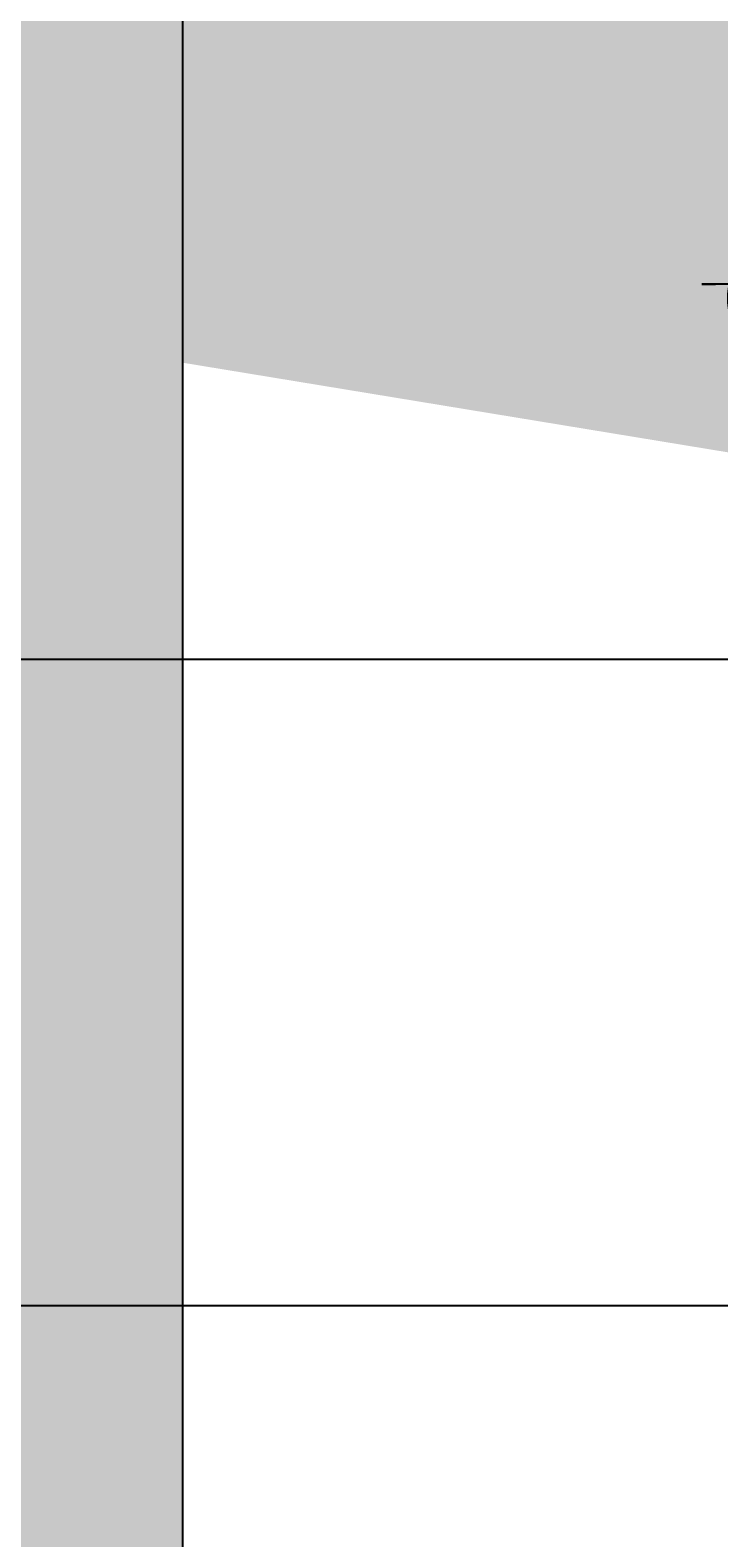
# Model space of a CAD drawing. Units: millimetres. Extents: x -22994 to 29398, y -19990 to 20176.
# Tile 52 of 135: x 198 to 216, y 25 to 65. Entities that reach past the tile are written whole.
import ezdxf
from ezdxf import colors
from ezdxf.entities.mleader import LeaderData, LeaderLine
from ezdxf.math import Vec2, Vec3

# ---------------------------------------------------------------- set-up
doc = ezdxf.new("R2010")
doc.units = ezdxf.units.MM
doc.header["$MEASUREMENT"] = 0
for name, color, linetype, lineweight in [('M-ANNO-TEXT', 7, 'Continuous', 25), ('M-DIMS', 2, 'Continuous', 18), ('M-EQPM', 7, 'Continuous', 25), ('M-EQPM-PATT', 7, 'Continuous', 18)]:
    doc.layers.add(name, color=color, linetype=linetype, lineweight=lineweight)
doc.styles.get("Standard").update_dxf_attribs({"font": 'arial.ttf'})
doc.dimstyles.get("Standard").update_dxf_attribs({"dimtxt": 0.18, "dimasz": 10000, "dimexe": 0.18, "dimexo": 0.0625, "dimgap": 0.09, "dimtad": 0, "dimtih": 1, "dimtoh": 1, "dimdec": 0, "dimzin": 0, "dimdsep": 46, "dimtxsty": 'Standard', "dimcen": 0.09, "dimadec": 0, "dimazin": 0, "dimtfac": 1, "dimtdec": 0, "dimtofl": 0, "dimtmove": 0, "dimatfit": 3, "dimfxl": 1, "dimtolj": 1, "dimtzin": 0, "dimlwd": 30, "dimarcsym": 0})

# ---------------------------------------------------------------- blocks, each defined once
blk = doc.blocks.new('*D2')
at = {"layer": 'Defpoints', "color": 0, "transparency": 16777216}
for p in [(6.677, 10.271), (290.852, 10.271), (290.852, -5.079)]:
    blk.add_point(p, dxfattribs=at)
at = {"layer": 'M-DIMS', "color": 0, "lineweight": -2, "transparency": 16777216}
for p, q in [((6.677, 10.209), (6.677, -5.259)), ((290.852, 10.209), (290.852, -5.259))]:
    blk.add_line(p, q, dxfattribs=at)
at = {"layer": 'M-DIMS', "color": 0, "lineweight": 30, "transparency": 16777216}
for p, q in [((-9993.323, -5.079), (-19993.323, -5.079)), ((10290.852, -5.079), (20290.852, -5.079))]:
    blk.add_line(p, q, dxfattribs=at)
at = {"layer": 'M-DIMS', "color": 0, "transparency": 16777216}
for points in [[(-9993.323, 1661.588), (-9993.323, -1671.745), (6.677, -5.079)], [(10290.852, 1661.588), (10290.852, -1671.745), (290.852, -5.079)]]:
    blk.add_solid(points, dxfattribs=at)
at = {"layer": 'M-DIMS', "color": 0, "transparency": 16777216, "insert": (148.765, -5.079), "char_height": 0.18, "attachment_point": 5}
blk.add_mtext('\\A1;284.2', dxfattribs=at)
blk = doc.blocks.new('*D3')
at = {"layer": 'Defpoints', "color": 0, "transparency": 16777216}
for p in [(110.265, 204.165), (110.265, 176.366), (95.833, 127.967)]:
    blk.add_point(p, dxfattribs=at)
at = {"layer": 'M-DIMS', "color": 0, "lineweight": -2, "transparency": 16777216}
for p, q in [((95.833, 128.03), (95.833, 204.345)), ((110.265, 176.429), (110.265, 204.345))]:
    blk.add_line(p, q, dxfattribs=at)
at = {"layer": 'M-DIMS', "color": 0, "lineweight": 30, "transparency": 16777216}
for p, q in [((-9904.167, 204.165), (-19904.167, 204.165)), ((10110.265, 204.165), (20110.265, 204.165))]:
    blk.add_line(p, q, dxfattribs=at)
at = {"layer": 'M-DIMS', "color": 0, "transparency": 16777216}
for points in [[(-9904.167, 1870.832), (-9904.167, -1462.501), (95.833, 204.165)], [(10110.265, 1870.832), (10110.265, -1462.501), (110.265, 204.165)]]:
    blk.add_solid(points, dxfattribs=at)
at = {"layer": 'M-DIMS', "color": 0, "transparency": 16777216, "insert": (103.049, 204.165), "char_height": 0.18, "attachment_point": 5}
blk.add_mtext('\\A1;14.432', dxfattribs=at)
blk = doc.blocks.new('*D4')
at = {"layer": 'Defpoints', "color": 0, "transparency": 16777216}
for p in [(116.265, 204.165), (110.265, 176.366), (116.265, 176.366)]:
    blk.add_point(p, dxfattribs=at)
at = {"layer": 'M-DIMS', "color": 0, "lineweight": -2, "transparency": 16777216}
for p, q in [((110.265, 176.429), (110.265, 204.345)), ((116.265, 176.429), (116.265, 204.345))]:
    blk.add_line(p, q, dxfattribs=at)
at = {"layer": 'M-DIMS', "color": 0, "lineweight": 30, "transparency": 16777216}
for p, q in [((-9889.735, 204.165), (-19889.735, 204.165)), ((10116.265, 204.165), (20116.265, 204.165))]:
    blk.add_line(p, q, dxfattribs=at)
at = {"layer": 'M-DIMS', "color": 0, "transparency": 16777216}
for points in [[(-9889.735, 1870.832), (-9889.735, -1462.501), (110.265, 204.165)], [(10116.265, 1870.832), (10116.265, -1462.501), (116.265, 204.165)]]:
    blk.add_solid(points, dxfattribs=at)
at = {"layer": 'M-DIMS', "color": 0, "transparency": 16777216, "insert": (113.265, 204.165), "char_height": 0.18, "attachment_point": 5}
blk.add_mtext('\\A1;6', dxfattribs=at)
blk = doc.blocks.new('*D5')
at = {"layer": 'Defpoints', "color": 0, "transparency": 16777216}
for p in [(181.265, 204.165), (116.265, 176.366), (181.265, 176.366)]:
    blk.add_point(p, dxfattribs=at)
at = {"layer": 'M-DIMS', "color": 0, "lineweight": -2, "transparency": 16777216}
for p, q in [((116.265, 176.429), (116.265, 204.345)), ((181.265, 176.429), (181.265, 204.345))]:
    blk.add_line(p, q, dxfattribs=at)
at = {"layer": 'M-DIMS', "color": 0, "lineweight": 30, "transparency": 16777216}
for p, q in [((-9883.735, 204.165), (-19883.735, 204.165)), ((10181.265, 204.165), (20181.265, 204.165))]:
    blk.add_line(p, q, dxfattribs=at)
at = {"layer": 'M-DIMS', "color": 0, "transparency": 16777216}
for points in [[(-9883.735, 1870.832), (-9883.735, -1462.501), (116.265, 204.165)], [(10181.265, 1870.832), (10181.265, -1462.501), (181.265, 204.165)]]:
    blk.add_solid(points, dxfattribs=at)
at = {"layer": 'M-DIMS', "color": 0, "transparency": 16777216, "insert": (148.765, 204.165), "char_height": 0.18, "attachment_point": 5}
blk.add_mtext('\\A1;65', dxfattribs=at)
blk = doc.blocks.new('*D6')
at = {"layer": 'Defpoints', "color": 0, "transparency": 16777216}
for p in [(187.265, 204.165), (181.265, 176.366), (187.265, 176.366)]:
    blk.add_point(p, dxfattribs=at)
at = {"layer": 'M-DIMS', "color": 0, "lineweight": -2, "transparency": 16777216}
for p, q in [((181.265, 176.429), (181.265, 204.345)), ((187.265, 176.429), (187.265, 204.345))]:
    blk.add_line(p, q, dxfattribs=at)
at = {"layer": 'M-DIMS', "color": 0, "lineweight": 30, "transparency": 16777216}
for p, q in [((-9818.735, 204.165), (-19818.735, 204.165)), ((10187.265, 204.165), (20187.265, 204.165))]:
    blk.add_line(p, q, dxfattribs=at)
at = {"layer": 'M-DIMS', "color": 0, "transparency": 16777216}
for points in [[(-9818.735, 1870.832), (-9818.735, -1462.501), (181.265, 204.165)], [(10187.265, 1870.832), (10187.265, -1462.501), (187.265, 204.165)]]:
    blk.add_solid(points, dxfattribs=at)
at = {"layer": 'M-DIMS', "color": 0, "transparency": 16777216, "insert": (184.265, 204.165), "char_height": 0.18, "attachment_point": 5}
blk.add_mtext('\\A1;6', dxfattribs=at)
blk = doc.blocks.new('*D7')
at = {"layer": 'Defpoints', "color": 0, "transparency": 16777216}
for p in [(201.697, 204.165), (187.265, 176.366), (201.697, 127.967)]:
    blk.add_point(p, dxfattribs=at)
at = {"layer": 'M-DIMS', "color": 0, "lineweight": -2, "transparency": 16777216}
for p, q in [((187.265, 176.429), (187.265, 204.345)), ((201.697, 128.03), (201.697, 204.345))]:
    blk.add_line(p, q, dxfattribs=at)
at = {"layer": 'M-DIMS', "color": 0, "lineweight": 30, "transparency": 16777216}
for p, q in [((-9812.735, 204.165), (-19812.735, 204.165)), ((10201.697, 204.165), (20201.697, 204.165))]:
    blk.add_line(p, q, dxfattribs=at)
at = {"layer": 'M-DIMS', "color": 0, "transparency": 16777216}
for points in [[(-9812.735, 1870.832), (-9812.735, -1462.501), (187.265, 204.165)], [(10201.697, 1870.832), (10201.697, -1462.501), (201.697, 204.165)]]:
    blk.add_solid(points, dxfattribs=at)
at = {"layer": 'M-DIMS', "color": 0, "transparency": 16777216, "insert": (194.481, 204.165), "char_height": 0.18, "attachment_point": 5}
blk.add_mtext('\\A1;14.432', dxfattribs=at)
blk = doc.blocks.new('*D8')
at = {"layer": 'Defpoints', "color": 0, "transparency": 16777216}
for p in [(227.648, 204.165), (227.648, 146.73), (201.697, 127.967)]:
    blk.add_point(p, dxfattribs=at)
at = {"layer": 'M-DIMS', "color": 0, "lineweight": -2, "transparency": 16777216}
for p, q in [((201.697, 128.03), (201.697, 204.345)), ((227.648, 146.792), (227.648, 204.345))]:
    blk.add_line(p, q, dxfattribs=at)
at = {"layer": 'M-DIMS', "color": 0, "lineweight": 30, "transparency": 16777216}
for p, q in [((-9798.303, 204.165), (-19798.303, 204.165)), ((10227.648, 204.165), (20227.648, 204.165))]:
    blk.add_line(p, q, dxfattribs=at)
at = {"layer": 'M-DIMS', "color": 0, "transparency": 16777216}
for points in [[(-9798.303, 1870.832), (-9798.303, -1462.501), (201.697, 204.165)], [(10227.648, 1870.832), (10227.648, -1462.501), (227.648, 204.165)]]:
    blk.add_solid(points, dxfattribs=at)
at = {"layer": 'M-DIMS', "color": 0, "transparency": 16777216, "insert": (214.673, 204.165), "char_height": 0.18, "attachment_point": 5}
blk.add_mtext('\\A1;25.95', dxfattribs=at)
blk = doc.blocks.new('*D9')
at = {"layer": 'Defpoints', "color": 0, "transparency": 16777216}
for p in [(187.265, 176.366), (306.202, 176.366), (290.852, 10.271)]:
    blk.add_point(p, dxfattribs=at)
at = {"layer": 'M-DIMS', "color": 0, "lineweight": 30, "transparency": 16777216}
for p, q in [((306.202, 10176.366), (306.202, 20176.366)), ((306.202, -9989.729), (306.202, -19989.729))]:
    blk.add_line(p, q, dxfattribs=at)
at = {"layer": 'M-DIMS', "color": 0, "lineweight": -2, "transparency": 16777216}
for p, q in [((187.327, 176.366), (306.382, 176.366)), ((290.915, 10.271), (306.382, 10.271))]:
    blk.add_line(p, q, dxfattribs=at)
at = {"layer": 'M-DIMS', "color": 0, "transparency": 16777216}
for points in [[(-1360.465, 10176.366), (1972.869, 10176.366), (306.202, 176.366)], [(-1360.465, -9989.729), (1972.869, -9989.729), (306.202, 10.271)]]:
    blk.add_solid(points, dxfattribs=at)
at = {"layer": 'M-DIMS', "color": 0, "transparency": 16777216, "insert": (306.202, 93.319), "char_height": 0.18, "attachment_point": 5}
blk.add_mtext('\\A1;166.1', dxfattribs=at)
blk = doc.blocks.new('*D10')
at = {"layer": 'Defpoints', "color": 0, "transparency": 16777216}
for p in [(125.65, 136.071), (133.346, 136.071), (133.346, -5.079)]:
    blk.add_point(p, dxfattribs=at)
at = {"layer": 'M-DIMS', "color": 0, "lineweight": -2, "transparency": 16777216}
for p, q in [((125.65, 136.009), (125.65, -5.259)), ((133.346, 136.009), (133.346, -5.259))]:
    blk.add_line(p, q, dxfattribs=at)
at = {"layer": 'M-DIMS', "color": 0, "lineweight": 30, "transparency": 16777216}
for p, q in [((-9874.35, -5.079), (-19874.35, -5.079)), ((10133.346, -5.079), (20133.346, -5.079))]:
    blk.add_line(p, q, dxfattribs=at)
at = {"layer": 'M-DIMS', "color": 0, "transparency": 16777216}
for points in [[(-9874.35, 1661.588), (-9874.35, -1671.745), (125.65, -5.079)], [(10133.346, 1661.588), (10133.346, -1671.745), (133.346, -5.079)]]:
    blk.add_solid(points, dxfattribs=at)
at = {"layer": 'M-DIMS', "color": 0, "transparency": 16777216, "insert": (129.498, -5.079), "char_height": 0.18, "attachment_point": 5}
blk.add_mtext('\\A1;7.696', dxfattribs=at)
blk = doc.blocks.new('*D11')
at = {"layer": 'Defpoints', "color": 0, "transparency": 16777216}
for p in [(133.346, 136.071), (135.65, 136.071), (135.65, -5.079)]:
    blk.add_point(p, dxfattribs=at)
at = {"layer": 'M-DIMS', "color": 0, "lineweight": -2, "transparency": 16777216}
for p, q in [((133.346, 136.009), (133.346, -5.259)), ((135.65, 136.009), (135.65, -5.259))]:
    blk.add_line(p, q, dxfattribs=at)
at = {"layer": 'M-DIMS', "color": 0, "lineweight": 30, "transparency": 16777216}
for p, q in [((-9866.654, -5.079), (-19866.654, -5.079)), ((10135.65, -5.079), (20135.65, -5.079))]:
    blk.add_line(p, q, dxfattribs=at)
at = {"layer": 'M-DIMS', "color": 0, "transparency": 16777216}
for points in [[(-9866.654, 1661.588), (-9866.654, -1671.745), (133.346, -5.079)], [(10135.65, 1661.588), (10135.65, -1671.745), (135.65, -5.079)]]:
    blk.add_solid(points, dxfattribs=at)
at = {"layer": 'M-DIMS', "color": 0, "transparency": 16777216, "insert": (134.498, -5.079), "char_height": 0.18, "attachment_point": 5}
blk.add_mtext('\\A1;2.304', dxfattribs=at)
blk = doc.blocks.new('*D12')
at = {"layer": 'Defpoints', "color": 0, "transparency": 16777216}
for p in [(135.65, 136.071), (145.65, 136.071), (145.65, -5.079)]:
    blk.add_point(p, dxfattribs=at)
at = {"layer": 'M-DIMS', "color": 0, "lineweight": -2, "transparency": 16777216}
for p, q in [((135.65, 136.009), (135.65, -5.259)), ((145.65, 136.009), (145.65, -5.259))]:
    blk.add_line(p, q, dxfattribs=at)
at = {"layer": 'M-DIMS', "color": 0, "lineweight": 30, "transparency": 16777216}
for p, q in [((-9864.35, -5.079), (-19864.35, -5.079)), ((10145.65, -5.079), (20145.65, -5.079))]:
    blk.add_line(p, q, dxfattribs=at)
at = {"layer": 'M-DIMS', "color": 0, "transparency": 16777216}
for points in [[(-9864.35, 1661.588), (-9864.35, -1671.745), (135.65, -5.079)], [(10145.65, 1661.588), (10145.65, -1671.745), (145.65, -5.079)]]:
    blk.add_solid(points, dxfattribs=at)
at = {"layer": 'M-DIMS', "color": 0, "transparency": 16777216, "insert": (140.65, -5.079), "char_height": 0.18, "attachment_point": 5}
blk.add_mtext('\\A1;10', dxfattribs=at)
blk = doc.blocks.new('*D13')
at = {"layer": 'Defpoints', "color": 0, "transparency": 16777216}
for p in [(145.65, 136.071), (155.65, 136.071), (155.65, -5.079)]:
    blk.add_point(p, dxfattribs=at)
at = {"layer": 'M-DIMS', "color": 0, "lineweight": -2, "transparency": 16777216}
for p, q in [((145.65, 136.009), (145.65, -5.259)), ((155.65, 136.009), (155.65, -5.259))]:
    blk.add_line(p, q, dxfattribs=at)
at = {"layer": 'M-DIMS', "color": 0, "lineweight": 30, "transparency": 16777216}
for p, q in [((-9854.35, -5.079), (-19854.35, -5.079)), ((10155.65, -5.079), (20155.65, -5.079))]:
    blk.add_line(p, q, dxfattribs=at)
at = {"layer": 'M-DIMS', "color": 0, "transparency": 16777216}
for points in [[(-9854.35, 1661.588), (-9854.35, -1671.745), (145.65, -5.079)], [(10155.65, 1661.588), (10155.65, -1671.745), (155.65, -5.079)]]:
    blk.add_solid(points, dxfattribs=at)
at = {"layer": 'M-DIMS', "color": 0, "transparency": 16777216, "insert": (150.65, -5.079), "char_height": 0.18, "attachment_point": 5}
blk.add_mtext('\\A1;10', dxfattribs=at)
blk = doc.blocks.new('*D14')
at = {"layer": 'Defpoints', "color": 0, "transparency": 16777216}
for p in [(155.65, 136.071), (165.65, 136.071), (165.65, -5.079)]:
    blk.add_point(p, dxfattribs=at)
at = {"layer": 'M-DIMS', "color": 0, "lineweight": -2, "transparency": 16777216}
for p, q in [((155.65, 136.009), (155.65, -5.259)), ((165.65, 136.009), (165.65, -5.259))]:
    blk.add_line(p, q, dxfattribs=at)
at = {"layer": 'M-DIMS', "color": 0, "lineweight": 30, "transparency": 16777216}
for p, q in [((-9844.35, -5.079), (-19844.35, -5.079)), ((10165.65, -5.079), (20165.65, -5.079))]:
    blk.add_line(p, q, dxfattribs=at)
at = {"layer": 'M-DIMS', "color": 0, "transparency": 16777216}
for points in [[(-9844.35, 1661.588), (-9844.35, -1671.745), (155.65, -5.079)], [(10165.65, 1661.588), (10165.65, -1671.745), (165.65, -5.079)]]:
    blk.add_solid(points, dxfattribs=at)
at = {"layer": 'M-DIMS', "color": 0, "transparency": 16777216, "insert": (160.65, -5.079), "char_height": 0.18, "attachment_point": 5}
blk.add_mtext('\\A1;10', dxfattribs=at)
blk = doc.blocks.new('*D15')
at = {"layer": 'Defpoints', "color": 0, "transparency": 16777216}
for p in [(173.346, 154.788), (173.346, 136.071), (306.202, 136.071)]:
    blk.add_point(p, dxfattribs=at)
at = {"layer": 'M-DIMS', "color": 0, "lineweight": 30, "transparency": 16777216}
for p, q in [((306.202, 10154.788), (306.202, 20154.788)), ((306.202, -9863.929), (306.202, -19863.929))]:
    blk.add_line(p, q, dxfattribs=at)
at = {"layer": 'M-DIMS', "color": 0, "lineweight": -2, "transparency": 16777216}
for p, q in [((173.408, 154.788), (306.382, 154.788)), ((173.408, 136.071), (306.382, 136.071))]:
    blk.add_line(p, q, dxfattribs=at)
at = {"layer": 'M-DIMS', "color": 0, "transparency": 16777216}
for points in [[(-1360.465, 10154.788), (1972.869, 10154.788), (306.202, 154.788)], [(-1360.465, -9863.929), (1972.869, -9863.929), (306.202, 136.071)]]:
    blk.add_solid(points, dxfattribs=at)
at = {"layer": 'M-DIMS', "color": 0, "transparency": 16777216, "insert": (306.202, 145.43), "char_height": 0.18, "attachment_point": 5}
blk.add_mtext('\\A1;18.717', dxfattribs=at)
blk = doc.blocks.new('*D16')
at = {"layer": 'Defpoints', "color": 0, "transparency": 16777216}
for p in [(120.17, 204.165), (110.466, 48.035), (120.17, 48.035)]:
    blk.add_point(p, dxfattribs=at)
at = {"layer": 'M-DIMS', "color": 0, "lineweight": -2, "transparency": 16777216}
for p, q in [((110.466, 48.097), (110.466, 204.345)), ((120.17, 48.097), (120.17, 204.345))]:
    blk.add_line(p, q, dxfattribs=at)
at = {"layer": 'M-DIMS', "color": 0, "lineweight": 30, "transparency": 16777216}
for p, q in [((-9889.534, 204.165), (-19889.534, 204.165)), ((10120.17, 204.165), (20120.17, 204.165))]:
    blk.add_line(p, q, dxfattribs=at)
at = {"layer": 'M-DIMS', "color": 0, "transparency": 16777216}
for points in [[(-9889.534, 1870.832), (-9889.534, -1462.501), (110.466, 204.165)], [(10120.17, 1870.832), (10120.17, -1462.501), (120.17, 204.165)]]:
    blk.add_solid(points, dxfattribs=at)
at = {"layer": 'M-DIMS', "color": 0, "transparency": 16777216, "insert": (115.318, 204.165), "char_height": 0.18, "attachment_point": 5}
blk.add_mtext('\\A1;9.704', dxfattribs=at)
blk = doc.blocks.new('*D17')
at = {"layer": 'Defpoints', "color": 0, "transparency": 16777216}
for p in [(126.17, 204.165), (120.17, 48.035), (126.17, 48.035)]:
    blk.add_point(p, dxfattribs=at)
at = {"layer": 'M-DIMS', "color": 0, "lineweight": -2, "transparency": 16777216}
for p, q in [((120.17, 48.097), (120.17, 204.345)), ((126.17, 48.097), (126.17, 204.345))]:
    blk.add_line(p, q, dxfattribs=at)
at = {"layer": 'M-DIMS', "color": 0, "lineweight": 30, "transparency": 16777216}
for p, q in [((-9879.83, 204.165), (-19879.83, 204.165)), ((10126.17, 204.165), (20126.17, 204.165))]:
    blk.add_line(p, q, dxfattribs=at)
at = {"layer": 'M-DIMS', "color": 0, "transparency": 16777216}
for points in [[(-9879.83, 1870.832), (-9879.83, -1462.501), (120.17, 204.165)], [(10126.17, 1870.832), (10126.17, -1462.501), (126.17, 204.165)]]:
    blk.add_solid(points, dxfattribs=at)
at = {"layer": 'M-DIMS', "color": 0, "transparency": 16777216, "insert": (123.17, 204.165), "char_height": 0.18, "attachment_point": 5}
blk.add_mtext('\\A1;6', dxfattribs=at)
blk = doc.blocks.new('*D18')
at = {"layer": 'Defpoints', "color": 0, "transparency": 16777216}
for p in [(132.17, 204.165), (126.17, 48.035), (132.17, 48.035)]:
    blk.add_point(p, dxfattribs=at)
at = {"layer": 'M-DIMS', "color": 0, "lineweight": -2, "transparency": 16777216}
for p, q in [((126.17, 48.097), (126.17, 204.345)), ((132.17, 48.097), (132.17, 204.345))]:
    blk.add_line(p, q, dxfattribs=at)
at = {"layer": 'M-DIMS', "color": 0, "lineweight": 30, "transparency": 16777216}
for p, q in [((-9873.83, 204.165), (-19873.83, 204.165)), ((10132.17, 204.165), (20132.17, 204.165))]:
    blk.add_line(p, q, dxfattribs=at)
at = {"layer": 'M-DIMS', "color": 0, "transparency": 16777216}
for points in [[(-9873.83, 1870.832), (-9873.83, -1462.501), (126.17, 204.165)], [(10132.17, 1870.832), (10132.17, -1462.501), (132.17, 204.165)]]:
    blk.add_solid(points, dxfattribs=at)
at = {"layer": 'M-DIMS', "color": 0, "transparency": 16777216, "insert": (129.17, 204.165), "char_height": 0.18, "attachment_point": 5}
blk.add_mtext('\\A1;6', dxfattribs=at)
blk = doc.blocks.new('*D19')
at = {"layer": 'Defpoints', "color": 0, "transparency": 16777216}
for p in [(138.17, 204.165), (132.17, 48.035), (138.17, 48.035)]:
    blk.add_point(p, dxfattribs=at)
at = {"layer": 'M-DIMS', "color": 0, "lineweight": -2, "transparency": 16777216}
for p, q in [((132.17, 48.097), (132.17, 204.345)), ((138.17, 48.097), (138.17, 204.345))]:
    blk.add_line(p, q, dxfattribs=at)
at = {"layer": 'M-DIMS', "color": 0, "lineweight": 30, "transparency": 16777216}
for p, q in [((-9867.83, 204.165), (-19867.83, 204.165)), ((10138.17, 204.165), (20138.17, 204.165))]:
    blk.add_line(p, q, dxfattribs=at)
at = {"layer": 'M-DIMS', "color": 0, "transparency": 16777216}
for points in [[(-9867.83, 1870.832), (-9867.83, -1462.501), (132.17, 204.165)], [(10138.17, 1870.832), (10138.17, -1462.501), (138.17, 204.165)]]:
    blk.add_solid(points, dxfattribs=at)
at = {"layer": 'M-DIMS', "color": 0, "transparency": 16777216, "insert": (135.17, 204.165), "char_height": 0.18, "attachment_point": 5}
blk.add_mtext('\\A1;6', dxfattribs=at)
blk = doc.blocks.new('*D20')
at = {"layer": 'Defpoints', "color": 0, "transparency": 16777216}
for p in [(144.17, 204.165), (138.17, 48.035), (144.17, 48.035)]:
    blk.add_point(p, dxfattribs=at)
at = {"layer": 'M-DIMS', "color": 0, "lineweight": -2, "transparency": 16777216}
for p, q in [((138.17, 48.097), (138.17, 204.345)), ((144.17, 48.097), (144.17, 204.345))]:
    blk.add_line(p, q, dxfattribs=at)
at = {"layer": 'M-DIMS', "color": 0, "lineweight": 30, "transparency": 16777216}
for p, q in [((-9861.83, 204.165), (-19861.83, 204.165)), ((10144.17, 204.165), (20144.17, 204.165))]:
    blk.add_line(p, q, dxfattribs=at)
at = {"layer": 'M-DIMS', "color": 0, "transparency": 16777216}
for points in [[(-9861.83, 1870.832), (-9861.83, -1462.501), (138.17, 204.165)], [(10144.17, 1870.832), (10144.17, -1462.501), (144.17, 204.165)]]:
    blk.add_solid(points, dxfattribs=at)
at = {"layer": 'M-DIMS', "color": 0, "transparency": 16777216, "insert": (141.17, 204.165), "char_height": 0.18, "attachment_point": 5}
blk.add_mtext('\\A1;6', dxfattribs=at)
blk = doc.blocks.new('*D21')
at = {"layer": 'Defpoints', "color": 0, "transparency": 16777216}
for p in [(149.116, 204.165), (144.17, 48.035), (149.116, 48.035)]:
    blk.add_point(p, dxfattribs=at)
at = {"layer": 'M-DIMS', "color": 0, "lineweight": -2, "transparency": 16777216}
for p, q in [((144.17, 48.097), (144.17, 204.345)), ((149.116, 48.097), (149.116, 204.345))]:
    blk.add_line(p, q, dxfattribs=at)
at = {"layer": 'M-DIMS', "color": 0, "lineweight": 30, "transparency": 16777216}
for p, q in [((-9855.83, 204.165), (-19855.83, 204.165)), ((10149.116, 204.165), (20149.116, 204.165))]:
    blk.add_line(p, q, dxfattribs=at)
at = {"layer": 'M-DIMS', "color": 0, "transparency": 16777216}
for points in [[(-9855.83, 1870.832), (-9855.83, -1462.501), (144.17, 204.165)], [(10149.116, 1870.832), (10149.116, -1462.501), (149.116, 204.165)]]:
    blk.add_solid(points, dxfattribs=at)
at = {"layer": 'M-DIMS', "color": 0, "transparency": 16777216, "insert": (146.643, 204.165), "char_height": 0.18, "attachment_point": 5}
blk.add_mtext('\\A1;4.945', dxfattribs=at)
blk = doc.blocks.new('*D22')
at = {"layer": 'Defpoints', "color": 0, "transparency": 16777216}
for p in [(149.116, 30.99), (155.116, 30.99), (155.116, -5.079)]:
    blk.add_point(p, dxfattribs=at)
at = {"layer": 'M-DIMS', "color": 0, "lineweight": -2, "transparency": 16777216}
for p, q in [((149.116, 30.927), (149.116, -5.259)), ((155.116, 30.927), (155.116, -5.259))]:
    blk.add_line(p, q, dxfattribs=at)
at = {"layer": 'M-DIMS', "color": 0, "lineweight": 30, "transparency": 16777216}
for p, q in [((-9850.884, -5.079), (-19850.884, -5.079)), ((10155.116, -5.079), (20155.116, -5.079))]:
    blk.add_line(p, q, dxfattribs=at)
at = {"layer": 'M-DIMS', "color": 0, "transparency": 16777216}
for points in [[(-9850.884, 1661.588), (-9850.884, -1671.745), (149.116, -5.079)], [(10155.116, 1661.588), (10155.116, -1671.745), (155.116, -5.079)]]:
    blk.add_solid(points, dxfattribs=at)
at = {"layer": 'M-DIMS', "color": 0, "transparency": 16777216, "insert": (152.116, -5.079), "char_height": 0.18, "attachment_point": 5}
blk.add_mtext('\\A1;6', dxfattribs=at)
blk = doc.blocks.new('*D23')
at = {"layer": 'Defpoints', "color": 0, "transparency": 16777216}
for p in [(155.116, 30.99), (161.116, 30.99), (161.116, -5.079)]:
    blk.add_point(p, dxfattribs=at)
at = {"layer": 'M-DIMS', "color": 0, "lineweight": -2, "transparency": 16777216}
for p, q in [((155.116, 30.927), (155.116, -5.259)), ((161.116, 30.927), (161.116, -5.259))]:
    blk.add_line(p, q, dxfattribs=at)
at = {"layer": 'M-DIMS', "color": 0, "lineweight": 30, "transparency": 16777216}
for p, q in [((-9844.884, -5.079), (-19844.884, -5.079)), ((10161.116, -5.079), (20161.116, -5.079))]:
    blk.add_line(p, q, dxfattribs=at)
at = {"layer": 'M-DIMS', "color": 0, "transparency": 16777216}
for points in [[(-9844.884, 1661.588), (-9844.884, -1671.745), (155.116, -5.079)], [(10161.116, 1661.588), (10161.116, -1671.745), (161.116, -5.079)]]:
    blk.add_solid(points, dxfattribs=at)
at = {"layer": 'M-DIMS', "color": 0, "transparency": 16777216, "insert": (158.116, -5.079), "char_height": 0.18, "attachment_point": 5}
blk.add_mtext('\\A1;6', dxfattribs=at)
blk = doc.blocks.new('*D24')
at = {"layer": 'Defpoints', "color": 0, "transparency": 16777216}
for p in [(161.116, 30.99), (166.439, 30.99), (166.439, -5.079)]:
    blk.add_point(p, dxfattribs=at)
at = {"layer": 'M-DIMS', "color": 0, "lineweight": -2, "transparency": 16777216}
for p, q in [((161.116, 30.927), (161.116, -5.259)), ((166.439, 30.927), (166.439, -5.259))]:
    blk.add_line(p, q, dxfattribs=at)
at = {"layer": 'M-DIMS', "color": 0, "lineweight": 30, "transparency": 16777216}
for p, q in [((-9838.884, -5.079), (-19838.884, -5.079)), ((10166.439, -5.079), (20166.439, -5.079))]:
    blk.add_line(p, q, dxfattribs=at)
at = {"layer": 'M-DIMS', "color": 0, "transparency": 16777216}
for points in [[(-9838.884, 1661.588), (-9838.884, -1671.745), (161.116, -5.079)], [(10166.439, 1661.588), (10166.439, -1671.745), (166.439, -5.079)]]:
    blk.add_solid(points, dxfattribs=at)
at = {"layer": 'M-DIMS', "color": 0, "transparency": 16777216, "insert": (163.777, -5.079), "char_height": 0.18, "attachment_point": 5}
blk.add_mtext('\\A1;5.323', dxfattribs=at)
blk = doc.blocks.new('*D25')
at = {"layer": 'Defpoints', "color": 0, "transparency": 16777216}
for p in [(166.439, 30.99), (172.439, 30.99), (172.439, -5.079)]:
    blk.add_point(p, dxfattribs=at)
at = {"layer": 'M-DIMS', "color": 0, "lineweight": -2, "transparency": 16777216}
for p, q in [((166.439, 30.927), (166.439, -5.259)), ((172.439, 30.927), (172.439, -5.259))]:
    blk.add_line(p, q, dxfattribs=at)
at = {"layer": 'M-DIMS', "color": 0, "lineweight": 30, "transparency": 16777216}
for p, q in [((-9833.561, -5.079), (-19833.561, -5.079)), ((10172.439, -5.079), (20172.439, -5.079))]:
    blk.add_line(p, q, dxfattribs=at)
at = {"layer": 'M-DIMS', "color": 0, "transparency": 16777216}
for points in [[(-9833.561, 1661.588), (-9833.561, -1671.745), (166.439, -5.079)], [(10172.439, 1661.588), (10172.439, -1671.745), (172.439, -5.079)]]:
    blk.add_solid(points, dxfattribs=at)
at = {"layer": 'M-DIMS', "color": 0, "transparency": 16777216, "insert": (169.439, -5.079), "char_height": 0.18, "attachment_point": 5}
blk.add_mtext('\\A1;6', dxfattribs=at)
blk = doc.blocks.new('*D26')
at = {"layer": 'Defpoints', "color": 0, "transparency": 16777216}
for p in [(172.439, 30.99), (178.439, 30.99), (178.439, -5.079)]:
    blk.add_point(p, dxfattribs=at)
at = {"layer": 'M-DIMS', "color": 0, "lineweight": -2, "transparency": 16777216}
for p, q in [((172.439, 30.927), (172.439, -5.259)), ((178.439, 30.927), (178.439, -5.259))]:
    blk.add_line(p, q, dxfattribs=at)
at = {"layer": 'M-DIMS', "color": 0, "lineweight": 30, "transparency": 16777216}
for p, q in [((-9827.561, -5.079), (-19827.561, -5.079)), ((10178.439, -5.079), (20178.439, -5.079))]:
    blk.add_line(p, q, dxfattribs=at)
at = {"layer": 'M-DIMS', "color": 0, "transparency": 16777216}
for points in [[(-9827.561, 1661.588), (-9827.561, -1671.745), (172.439, -5.079)], [(10178.439, 1661.588), (10178.439, -1671.745), (178.439, -5.079)]]:
    blk.add_solid(points, dxfattribs=at)
at = {"layer": 'M-DIMS', "color": 0, "transparency": 16777216, "insert": (175.439, -5.079), "char_height": 0.18, "attachment_point": 5}
blk.add_mtext('\\A1;6', dxfattribs=at)
blk = doc.blocks.new('*D27')
at = {"layer": 'Defpoints', "color": 0, "transparency": 16777216}
for p in [(178.439, 30.99), (188.117, 30.99), (188.117, -5.079)]:
    blk.add_point(p, dxfattribs=at)
at = {"layer": 'M-DIMS', "color": 0, "lineweight": -2, "transparency": 16777216}
for p, q in [((178.439, 30.927), (178.439, -5.259)), ((188.117, 30.927), (188.117, -5.259))]:
    blk.add_line(p, q, dxfattribs=at)
at = {"layer": 'M-DIMS', "color": 0, "lineweight": 30, "transparency": 16777216}
for p, q in [((-9821.561, -5.079), (-19821.561, -5.079)), ((10188.117, -5.079), (20188.117, -5.079))]:
    blk.add_line(p, q, dxfattribs=at)
at = {"layer": 'M-DIMS', "color": 0, "transparency": 16777216}
for points in [[(-9821.561, 1661.588), (-9821.561, -1671.745), (178.439, -5.079)], [(10188.117, 1661.588), (10188.117, -1671.745), (188.117, -5.079)]]:
    blk.add_solid(points, dxfattribs=at)
at = {"layer": 'M-DIMS', "color": 0, "transparency": 16777216, "insert": (183.278, -5.079), "char_height": 0.18, "attachment_point": 5}
blk.add_mtext('\\A1;9.679', dxfattribs=at)
blk = doc.blocks.new('*D28')
at = {"layer": 'Defpoints', "color": 0, "transparency": 16777216}
for p in [(188.117, 48.035), (306.202, 48.035), (188.117, 30.99)]:
    blk.add_point(p, dxfattribs=at)
at = {"layer": 'M-DIMS', "color": 0, "lineweight": 30, "transparency": 16777216}
for p, q in [((306.202, 10048.035), (306.202, 20048.035)), ((306.202, -9969.01), (306.202, -19969.01))]:
    blk.add_line(p, q, dxfattribs=at)
at = {"layer": 'M-DIMS', "color": 0, "lineweight": -2, "transparency": 16777216}
for p, q in [((188.18, 48.035), (306.382, 48.035)), ((188.18, 30.99), (306.382, 30.99))]:
    blk.add_line(p, q, dxfattribs=at)
at = {"layer": 'M-DIMS', "color": 0, "transparency": 16777216}
for points in [[(-1360.465, 10048.035), (1972.869, 10048.035), (306.202, 48.035)], [(-1360.465, -9969.01), (1972.869, -9969.01), (306.202, 30.99)]]:
    blk.add_solid(points, dxfattribs=at)
at = {"layer": 'M-DIMS', "color": 0, "transparency": 16777216, "insert": (306.202, 39.512), "char_height": 0.18, "attachment_point": 5}
blk.add_mtext('\\A1;17.045', dxfattribs=at)
blk = doc.blocks.new('*D29')
at = {"layer": 'Defpoints', "color": 0, "transparency": 16777216}
for p in [(36.801, 80.045), (64.03, 80.045)]:
    blk.add_point(p, dxfattribs=at)
at = {"layer": 'M-DIMS', "color": 0, "lineweight": -2, "transparency": 16777216}
for p, q in [((50.325, 80.045), (50.505, 80.045)), ((50.415, 79.955), (50.415, 80.135))]:
    blk.add_line(p, q, dxfattribs=at)
at = {"layer": 'M-DIMS', "color": 0, "lineweight": 30, "transparency": 16777216}
blk.add_line((20064.03, 80.03), (10064.03, 80.038), dxfattribs=at)
at = {"layer": 'M-DIMS', "color": 0, "transparency": 16777216}
blk.add_solid([(10064.031, 1746.704), (10064.028, -1586.629), (64.03, 80.045)], dxfattribs=at)
at = {"layer": 'M-DIMS', "color": 0, "transparency": 16777216, "insert": (20064.521, 80.03), "char_height": 0.18, "attachment_point": 5}
blk.add_mtext('\\A1;∅27.23', dxfattribs=at)
blk = doc.blocks.new('*D36')
at = {"layer": 'Defpoints', "color": 0, "transparency": 16777216}
for p in [(46.39, 31.303), (46.387, 26.593)]:
    blk.add_point(p, dxfattribs=at)
at = {"layer": 'M-DIMS', "color": 0, "lineweight": 30, "transparency": 16777216}
for p, q in [((57.15, 20031.301), (51.77, 10031.302)), ((10057.15, 20031.301), (57.15, 20031.301))]:
    blk.add_line(p, q, dxfattribs=at)
at = {"layer": 'M-DIMS', "color": 0, "lineweight": -2, "transparency": 16777216}
for p, q in [((46.389, 28.858), (46.389, 29.038)), ((46.299, 28.948), (46.479, 28.948))]:
    blk.add_line(p, q, dxfattribs=at)
at = {"layer": 'M-DIMS', "color": 0, "transparency": 16777216}
blk.add_solid([(-1614.896, 10032.199), (1718.436, 10030.405), (46.39, 31.303)], dxfattribs=at)
at = {"layer": 'M-DIMS', "color": 0, "transparency": 16777216, "insert": (10057.554, 20031.301), "char_height": 0.18, "attachment_point": 5}
blk.add_mtext('\\A1;∅4.71', dxfattribs=at)
blk = doc.blocks.new('*D37')
at = {"layer": 'Defpoints', "color": 0, "transparency": 16777216}
for p in [(54.834, 118.615), (59.494, 118.614)]:
    blk.add_point(p, dxfattribs=at)
at = {"layer": 'M-DIMS', "color": 0, "lineweight": -2, "transparency": 16777216}
for p, q in [((57.074, 118.614), (57.254, 118.614)), ((57.164, 118.524), (57.164, 118.704))]:
    blk.add_line(p, q, dxfattribs=at)
at = {"layer": 'M-DIMS', "color": 0, "lineweight": 30, "transparency": 16777216}
blk.add_line((20059.493, 116.253), (10059.494, 117.434), dxfattribs=at)
at = {"layer": 'M-DIMS', "color": 0, "transparency": 16777216}
blk.add_solid([(10059.69, 1784.1), (10059.297, -1549.233), (59.494, 118.614)], dxfattribs=at)
at = {"layer": 'M-DIMS', "color": 0, "transparency": 16777216, "insert": (20059.985, 116.253), "char_height": 0.18, "attachment_point": 5}
blk.add_mtext('\\A1;∅4.659', dxfattribs=at)

msp = doc.modelspace()

# ---------------------------------------------------------------- hatches: boundary and pattern name
at = {"layer": 'M-EQPM-PATT'}
h = msp.add_hatch(color=256, dxfattribs=at)
h.set_gradient(color1=(205, 32, 39), color2=(205, 32, 39), tint=1)
h.paths.add_polyline_path([(116.2647, 150.3662), (116.2647, 170.3662), (116.2647, 176.3662), (110.2647, 176.3662), (110.2647, 152.0276), (95.8327, 127.967), (95.8327, 16.6063), (201.6967, 16.6063), (201.6967, 127.967), (187.2647, 152.0276), (187.2647, 176.3662), (181.2647, 176.3662), (181.2647, 170.3662), (181.2647, 150.3662), (195.6967, 126.3055), (195.6967, 22.6063), (101.8327, 22.6063), (101.8327, 126.3055)])
h.paths.add_polyline_path([(185.2208, 88.6347), (101.8327, 88.6347), (101.8327, 87.6347), (182.8066, 87.6347), (178.7313, 83.5594), (195.6967, 83.5594), (195.6967, 84.5594), (181.1455, 84.5594)], flags=17)
h.paths.add_polyline_path([(95.8327, 88.6347), (60.9779, 88.6347, -0.0228552), (61.7178, 87.6347), (95.8327, 87.6347)])
h.paths.add_polyline_path([(215.6212, 86.5189), (215.6212, 80.5999), (220.5095, 83.5594)])
h.paths.add_polyline_path([(215.6212, 84.5594), (201.6967, 84.5594), (201.6967, 83.5594), (215.6212, 83.5594)])
h.paths.add_polyline_path([(225.3978, 86.5189), (220.5095, 83.5594), (225.3978, 80.5999)])
h.paths.add_polyline_path([(231.6256, 84.5594), (225.3978, 84.5594), (225.3978, 83.5594), (231.6256, 83.5594)])

# ---------------------------------------------------------------- linework, layer by layer
at = {"layer": 'M-EQPM'}
msp.add_lwpolyline([(110.2647, 176.3662), (110.2647, 152.0276), (95.8327, 127.967), (95.8327, 16.6063), (201.6967, 16.6063), (201.6967, 127.967), (187.2647, 152.0276), (187.2647, 176.3662)], close=True, dxfattribs=at)

# ---------------------------------------------------------------- dimensions: what is measured, and where the dimension line sits
at = {"layer": 'M-DIMS'}
for base, p1, p2, override, picture, middle in [((306.202, 176.3662), (290.852, 10.2713), (187.2647, 176.3662), {"dimdec": 1, "dimlfac": 1, "dimrnd": 0, "dimzin": 0, "dimdsep": 46, "dimlunit": 2}, '*D9', (306.202, 93.3187)), ((306.202, 136.0713), (173.3459, 154.788), (173.3459, 136.0713), {"dimdec": 3, "dimlfac": 1, "dimrnd": 0, "dimzin": 0, "dimdsep": 46, "dimlunit": 2}, '*D15', (306.202, 145.4297)), ((306.202, 48.0349), (188.1175, 30.9895), (188.1175, 48.0349), {"dimdec": 3, "dimlfac": 1, "dimrnd": 0, "dimzin": 0, "dimdsep": 46, "dimlunit": 2}, '*D28', (306.202, 39.5122))]:
    dim = msp.add_linear_dim(base=base, p1=p1, p2=p2, angle=90, dimstyle='Standard', override=override, dxfattribs=at)
    dim.commit()
    dim.dimension.update_dxf_attribs({"geometry": picture, "text_midpoint": middle})
dim = msp.add_diameter_dim_2p(p1=(46.3875, 26.5934), p2=(46.39, 31.3035), dimstyle='Standard', override={"dimdec": 2, "dimlfac": 1, "dimrnd": 0, "dimzin": 0, "dimdsep": 46, "dimlunit": 2}, dxfattribs=at)
dim.commit()
dim.dimension.update_dxf_attribs({"geometry": '*D36', "text_midpoint": (10057.5542, 20031.3006), "dimtype": 163})
for base, p1, p2, override, picture, middle in [((110.2647, 204.1654), (95.8327, 127.967), (110.2647, 176.3662), {"dimdec": 3, "dimlfac": 1, "dimrnd": 0, "dimzin": 0, "dimdsep": 46, "dimlunit": 2}, '*D3', (103.0487, 204.1654)), ((116.2647, 204.1654), (110.2647, 176.3662), (116.2647, 176.3662), {"dimdec": 0, "dimlfac": 1, "dimrnd": 0, "dimzin": 0, "dimdsep": 46, "dimlunit": 2}, '*D4', (113.2647, 204.1654)), ((120.1702, 204.1654), (110.4658, 48.0349), (120.1702, 48.0349), {"dimdec": 3, "dimlfac": 1, "dimrnd": 0, "dimzin": 0, "dimdsep": 46, "dimlunit": 2}, '*D16', (115.318, 204.1654)), ((181.2647, 204.1654), (116.2647, 176.3662), (181.2647, 176.3662), {"dimdec": 0, "dimlfac": 1, "dimrnd": 0, "dimzin": 0, "dimdsep": 46, "dimlunit": 2}, '*D5', (148.7647, 204.1654)), ((126.1702, 204.1654), (120.1702, 48.0349), (126.1702, 48.0349), {"dimdec": 0, "dimlfac": 1, "dimrnd": 0, "dimzin": 0, "dimdsep": 46, "dimlunit": 2}, '*D17', (123.1702, 204.1654)), ((132.1702, 204.1654), (126.1702, 48.0349), (132.1702, 48.0349), {"dimdec": 0, "dimlfac": 1, "dimrnd": 0, "dimzin": 0, "dimdsep": 46, "dimlunit": 2}, '*D18', (129.1702, 204.1654)), ((138.1702, 204.1654), (132.1702, 48.0349), (138.1702, 48.0349), {"dimdec": 0, "dimlfac": 1, "dimrnd": 0, "dimzin": 0, "dimdsep": 46, "dimlunit": 2}, '*D19', (135.1702, 204.1654)), ((144.1702, 204.1654), (138.1702, 48.0349), (144.1702, 48.0349), {"dimdec": 0, "dimlfac": 1, "dimrnd": 0, "dimzin": 0, "dimdsep": 46, "dimlunit": 2}, '*D20', (141.1702, 204.1654)), ((149.11567, 204.16539), (144.17023, 48.03494), (149.11567, 48.03494), {"dimdec": 3, "dimlfac": 1, "dimrnd": 0, "dimzin": 0, "dimdsep": 46, "dimlunit": 2}, '*D21', (146.64295, 204.16539)), ((187.2647, 204.1654), (181.2647, 176.3662), (187.2647, 176.3662), {"dimdec": 0, "dimlfac": 1, "dimrnd": 0, "dimzin": 0, "dimdsep": 46, "dimlunit": 2}, '*D6', (184.2647, 204.1654)), ((201.6967, 204.1654), (187.2647, 176.3662), (201.6967, 127.967), {"dimdec": 3, "dimlfac": 1, "dimrnd": 0, "dimzin": 0, "dimdsep": 46, "dimlunit": 2}, '*D7', (194.4807, 204.1654)), ((227.6485, 204.1654), (201.6967, 127.967), (227.6485, 146.7296), {"dimdec": 2, "dimlfac": 1, "dimrnd": 0, "dimzin": 0, "dimdsep": 46, "dimlunit": 2}, '*D8', (214.6726, 204.1654)), ((290.852, -5.0787), (6.6773, 10.2713), (290.852, 10.2713), {"dimdec": 1, "dimlfac": 1, "dimrnd": 0, "dimzin": 0, "dimdsep": 46, "dimlunit": 2}, '*D2', (148.7647, -5.0787)), ((133.3459, -5.0787), (125.6498, 136.0713), (133.3459, 136.0713), {"dimdec": 3, "dimlfac": 1, "dimrnd": 0, "dimzin": 0, "dimdsep": 46, "dimlunit": 2}, '*D10', (129.4978, -5.0787)), ((135.6498, -5.0787), (133.3459, 136.0713), (135.6498, 136.0713), {"dimdec": 3, "dimlfac": 1, "dimrnd": 0, "dimzin": 0, "dimdsep": 46, "dimlunit": 2}, '*D11', (134.4978, -5.0787)), ((145.6498, -5.0787), (135.6498, 136.0713), (145.6498, 136.0713), {"dimdec": 0, "dimlfac": 1, "dimrnd": 0, "dimzin": 0, "dimdsep": 46, "dimlunit": 2}, '*D12', (140.6498, -5.0787)), ((155.6498, -5.0787), (145.6498, 136.0713), (155.6498, 136.0713), {"dimdec": 0, "dimlfac": 1, "dimrnd": 0, "dimzin": 0, "dimdsep": 46, "dimlunit": 2}, '*D13', (150.6498, -5.0787)), ((155.1157, -5.0787), (149.1157, 30.9895), (155.1157, 30.9895), {"dimdec": 0, "dimlfac": 1, "dimrnd": 0, "dimzin": 0, "dimdsep": 46, "dimlunit": 2}, '*D22', (152.1157, -5.0787)), ((161.1157, -5.0787), (155.1157, 30.9895), (161.1157, 30.9895), {"dimdec": 0, "dimlfac": 1, "dimrnd": 0, "dimzin": 0, "dimdsep": 46, "dimlunit": 2}, '*D23', (158.1157, -5.0787)), ((165.6498, -5.0787), (155.6498, 136.0713), (165.6498, 136.0713), {"dimdec": 0, "dimlfac": 1, "dimrnd": 0, "dimzin": 0, "dimdsep": 46, "dimlunit": 2}, '*D14', (160.6498, -5.0787)), ((166.4387, -5.0787), (161.1157, 30.9895), (166.4387, 30.9895), {"dimdec": 3, "dimlfac": 1, "dimrnd": 0, "dimzin": 0, "dimdsep": 46, "dimlunit": 2}, '*D24', (163.7772, -5.0787)), ((172.4387, -5.0787), (166.4387, 30.9895), (172.4387, 30.9895), {"dimdec": 0, "dimlfac": 1, "dimrnd": 0, "dimzin": 0, "dimdsep": 46, "dimlunit": 2}, '*D25', (169.4387, -5.0787)), ((178.4387, -5.0787), (172.4387, 30.9895), (178.4387, 30.9895), {"dimdec": 0, "dimlfac": 1, "dimrnd": 0, "dimzin": 0, "dimdsep": 46, "dimlunit": 2}, '*D26', (175.4387, -5.0787)), ((188.1175, -5.0787), (178.4387, 30.9895), (188.1175, 30.9895), {"dimdec": 3, "dimlfac": 1, "dimrnd": 0, "dimzin": 0, "dimdsep": 46, "dimlunit": 2}, '*D27', (183.2781, -5.0787))]:
    dim = msp.add_linear_dim(base=base, p1=p1, p2=p2, dimstyle='Standard', override=override, dxfattribs=at)
    dim.commit()
    dim.dimension.update_dxf_attribs({"geometry": picture, "text_midpoint": middle})
for p1, p2, override, picture, middle in [((54.8343, 118.6145), (59.4936, 118.614), {"dimdec": 3, "dimlfac": 1, "dimrnd": 0, "dimzin": 0, "dimdsep": 46, "dimlunit": 2}, '*D37', (20059.4934, 116.2531)), ((36.8006, 80.045), (64.0296, 80.045), {"dimdec": 2, "dimlfac": 1, "dimrnd": 0, "dimzin": 0, "dimdsep": 46, "dimlunit": 2}, '*D29', (20064.0296, 80.0303))]:
    dim = msp.add_diameter_dim_2p(p1=p1, p2=p2, dimstyle='Standard', override=override, dxfattribs=at)
    dim.commit()
    dim.dimension.update_dxf_attribs({"geometry": picture, "text_midpoint": middle})

# ---------------------------------------------------------------- leaders
at = {"layer": 'M-ANNO-TEXT'}
ml = msp.add_multileader_mtext('Standard', dxfattribs=at)
ml.set_content('combustion chamber', color=256)
ml.set_leader_properties()
ml.build(insert=Vec2(0, 0))
ml.multileader.update_dxf_attribs({"dogleg_length": 0.36, "arrow_head_size": 200})
ctx = ml.context
ctx.base_point, ctx.char_height, ctx.arrow_head_size, ctx.landing_gap_size, ctx.plane_origin = Vec3(215.7321, 57.9149), 3, 200, 0.09, Vec3(189.1175, 57.9149)
notes = []
notes.append((ctx, [(0, (1, 1, 0), (215.3721, 57.9149), (1, 0), 0.36, [(0, [(189.1175, 57.9149)], 0, [])])]))
ctx.mtext.insert, ctx.mtext.flow_direction = Vec3(215.8221, 59.4394), 5
for ctx, leaders in notes:
    for number, flags, end, landing, length, lines in leaders:
        leader = LeaderData()
        leader.index, (leader.has_last_leader_line, leader.has_dogleg_vector, leader.attachment_direction) = number, flags
        leader.last_leader_point, leader.dogleg_vector, leader.dogleg_length = Vec3(end), Vec3(landing), length
        for number, points, colour, breaks in lines:
            line = LeaderLine()
            line.index, line.vertices, line.color, line.breaks = number, Vec3.list(points), colors.encode_raw_color(colour), breaks
            leader.lines.append(line)
        ctx.leaders.append(leader)

doc.saveas('drawing.dxf')
